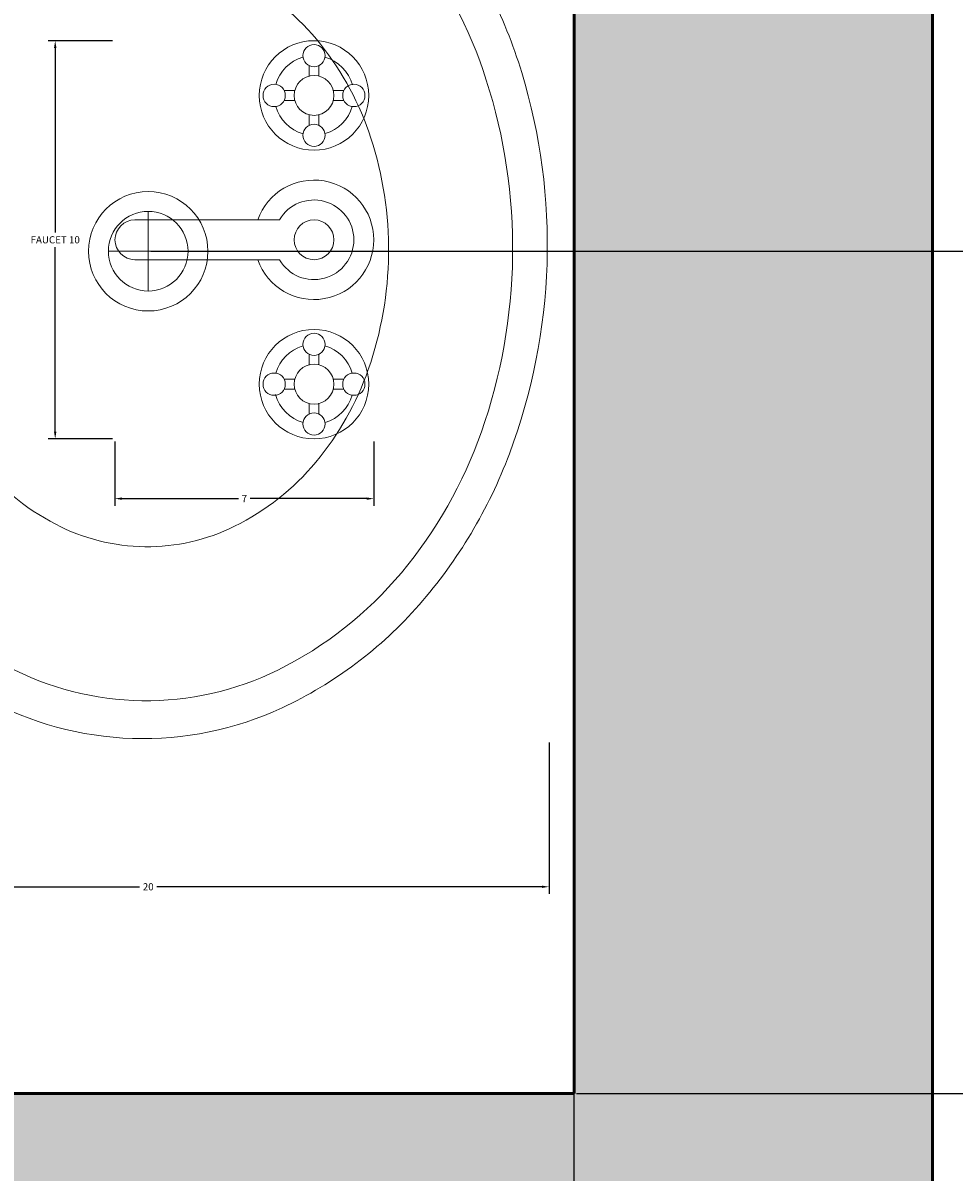
# Model space of a CAD drawing. Units: inches. Extents: x 2307 to 2544, y 2171 to 2540.
# Tile 42 of 52: x 2502 to 2525, y 2438 to 2466. Entities that reach past the tile are written whole.
import ezdxf

# ---------------------------------------------------------------- set-up
doc = ezdxf.new("R2010")
doc.units = ezdxf.units.IN
for name, color, linetype, lineweight in [('A-ANNO-DIMS', 2, 'Continuous', 18), ('A-FLOR-FIXT', 9, 'Continuous', 18), ('A-WALL', 7, 'Continuous', 50)]:
    doc.layers.add(name, color=color, linetype=linetype, lineweight=lineweight)
doc.layers.add('A-WALL-PATT', color=18, linetype='Continuous', lineweight=13, true_color=0x000000)
doc.styles.get("Standard").update_dxf_attribs({"font": 'arial.ttf'})
doc.dimstyles.get("Standard").update_dxf_attribs({"dimtxt": 0.18, "dimasz": 0.18, "dimexe": 0.18, "dimexo": 0.0625, "dimgap": 0.09, "dimtad": 0, "dimtih": 1, "dimtoh": 1, "dimdec": 4, "dimzin": 0, "dimdsep": 46, "dimtxsty": 'Standard', "dimcen": 0.09, "dimadec": 0, "dimazin": 0, "dimtfac": 1, "dimtdec": 4, "dimtofl": 0, "dimtmove": 0, "dimatfit": 3, "dimfxl": 1, "dimtolj": 1, "dimtzin": 0, "dimarcsym": 0})

# ---------------------------------------------------------------- blocks, each defined once
blk = doc.blocks.new('Sink - Oval top')
for p, q in [((0, 1), (0, -1)), ((-1, 0), (1, 0))]:
    blk.add_line(p, q)
for points in [[(-12.234, 0.394, 0.117634), (-11.465, -3.362, 0.104469), (-8.879, -6.804, 0.090016), (-5.083, -9.072, 0.08192), (-0.323, -10.016, 0.08192), (4.488, -9.381, 0.090016), (8.422, -7.361, 0.104469), (11.224, -4.093, 0.117634), (12.234, -0.394, 0.117634), (11.465, 3.362, 0.104469), (8.879, 6.804, 0.090016), (5.083, 9.072, 0.08192), (0.323, 10.016, 0.08192), (-4.488, 9.381, 0.090016), (-8.422, 7.361, 0.104469), (-11.224, 4.093, 0.117634)], [(-11.286, 0.159, 0.118622), (-10.516, -3.253, 0.104678), (-8.072, -6.359, 0.089562), (-4.538, -8.367, 0.081185), (-0.129, -9.152, 0.081185), (4.3, -8.492, 0.089562), (7.889, -6.584, 0.104678), (10.42, -3.548, 0.118622), (11.286, -0.159, 0.118622), (10.516, 3.253, 0.104678), (8.072, 6.359, 0.089562), (4.538, 8.367, 0.081185), (0.129, 9.152, 0.081185), (-4.3, 8.492, 0.089562), (-7.889, 6.584, 0.104678), (-10.42, 3.548, 0.118622)], [(-7.42, 0.083, 0.118283), (-6.907, -2.167, 0.104607), (-5.295, -4.21, 0.089718), (-2.967, -5.528, 0.081436), (-0.068, -6.037, 0.081436), (2.842, -5.593, 0.089718), (5.199, -4.327, 0.104607), (6.857, -2.321, 0.118283), (7.42, -0.083, 0.118283), (6.907, 2.167, 0.104607), (5.295, 4.21, 0.089718), (2.967, 5.528, 0.081436), (0.068, 6.037, 0.081436), (-2.842, 5.593, 0.089718), (-5.199, 4.327, 0.104607), (-6.857, 2.321, 0.118283)]]:
    blk.add_lwpolyline(points, format="xyb", close=True)
for radius in [1.5, 1]:
    blk.add_circle((0, 0), radius)
blk = doc.blocks.new('Faucet - Bathroom top')
for p, q in [((-3.75, 0.4788), (-3.75, 0.75)), ((-3.5, 0.482), (-3.5, 0.75)), ((3.5, 0.4788), (3.5, 0.75)), ((3.75, 0.482), (3.75, 0.75)), ((-4.107, 0.125), (-4.375, 0.125)), ((-3.1461, 0.125), (-2.875, 0.125)), ((3.143, 0.125), (2.875, 0.125)), ((4.1039, 0.125), (4.375, 0.125)), ((-4.1039, -0.125), (-4.375, -0.125)), ((-3.143, -0.125), (-2.875, -0.125)), ((3.1461, -0.125), (2.875, -0.125)), ((4.107, -0.125), (4.375, -0.125)), ((-3.75, -0.4821), (-3.75, -0.75)), ((-3.5, -0.4789), (-3.5, -0.75)), ((3.5, -0.4821), (3.5, -0.75)), ((3.75, -0.4789), (3.75, -0.75)), ((-0.5, -0.8639), (-0.5, -4.5)), ((0.5, -4.5), (0.5, -0.8631))]:
    blk.add_line(p, q)
for centre, radius in [((-3.625, 0), 1.375), ((-3.625, 1), 0.2795), ((3.625, 0), 1.375), ((3.625, 1), 0.2795), ((-3.625, 0), 0.5), ((0, 0), 0.5), ((3.625, 0), 0.5), ((-4.625, 0), 0.2795), ((-2.625, 0), 0.2795), ((2.625, 0), 0.2795), ((4.625, 0), 0.2795), ((-3.625, -1), 0.2795), ((3.625, -1), 0.2795)]:
    blk.add_circle(centre, radius)
for centre, radius, start, end in [((0, 0), 1.5, 289.6514, 250.3603), ((-3.625, 0), 1, 105.2407, 164.2093), ((-3.625, 0), 1, 16.44125, 74.07887), ((0, 0), 1, 300.3431, 239.7554), ((3.625, 0), 1, 106.12, 164.0884), ((3.625, 0), 1, 16.23422, 73.90469), ((-3.625, 0), 1, 196.2342, 253.9047), ((-3.625, 0), 1, 286.12, 344.0884), ((3.625, 0), 1, 196.4413, 254.0789), ((3.625, 0), 1, 285.2407, 344.2093), ((0, -4.5), 0.5, 180, 0)]:
    blk.add_arc(centre, radius, start, end)
blk = doc.blocks.new('*D23')
at = {"layer": 'A-ANNO-DIMS', "color": 0, "lineweight": -2, "transparency": 16777216}
for p, q in [((2494.934, 2448.317), (2494.934, 2444.517)), ((2515.07, 2448.317), (2515.07, 2444.517)), ((2495.114, 2444.697), (2504.782, 2444.697)), ((2514.89, 2444.697), (2505.222, 2444.697))]:
    blk.add_line(p, q, dxfattribs=at)
at = {"layer": 'A-ANNO-DIMS', "color": 0, "transparency": 16777216}
for points in [[(2495.114, 2444.727), (2495.114, 2444.667), (2494.934, 2444.697)], [(2514.89, 2444.727), (2514.89, 2444.667), (2515.07, 2444.697)]]:
    blk.add_solid(points, dxfattribs=at)
at = {"layer": 'Defpoints', "color": 0, "transparency": 16777216}
for p in [(2494.934, 2448.38), (2515.07, 2448.38), (2515.07, 2444.697)]:
    blk.add_point(p, dxfattribs=at)
at = {"layer": 'A-ANNO-DIMS', "color": 0, "transparency": 16777216, "insert": (2505.002, 2444.697), "char_height": 0.18, "attachment_point": 5}
blk.add_mtext('\\A1;20', dxfattribs=at)
blk = doc.blocks.new('*D24')
at = {"layer": 'A-ANNO-DIMS', "color": 0, "lineweight": -2, "transparency": 16777216}
for p, q in [((2504.104, 2465.943), (2502.486, 2465.943)), ((2502.666, 2465.763), (2502.666, 2461.126)), ((2502.666, 2456.123), (2502.666, 2460.76)), ((2504.104, 2455.943), (2502.486, 2455.943))]:
    blk.add_line(p, q, dxfattribs=at)
at = {"layer": 'A-ANNO-DIMS', "color": 0, "transparency": 16777216}
for points in [[(2502.636, 2465.763), (2502.696, 2465.763), (2502.666, 2465.943)], [(2502.636, 2456.123), (2502.696, 2456.123), (2502.666, 2455.943)]]:
    blk.add_solid(points, dxfattribs=at)
at = {"layer": 'Defpoints', "color": 0, "transparency": 16777216}
for p in [(2504.166, 2465.943), (2502.666, 2455.943), (2504.166, 2455.943)]:
    blk.add_point(p, dxfattribs=at)
at = {"layer": 'A-ANNO-DIMS', "color": 0, "transparency": 16777216, "insert": (2502.666, 2460.943), "char_height": 0.18, "attachment_point": 5}
blk.add_mtext('\\A1;FAUCET 10', dxfattribs=at)
blk = doc.blocks.new('*D25')
at = {"layer": 'A-ANNO-DIMS', "color": 0, "lineweight": -2, "transparency": 16777216}
for p, q in [((2504.166, 2455.88), (2504.166, 2454.263)), ((2510.666, 2455.88), (2510.666, 2454.263)), ((2504.346, 2454.443), (2507.268, 2454.443)), ((2510.486, 2454.443), (2507.565, 2454.443))]:
    blk.add_line(p, q, dxfattribs=at)
at = {"layer": 'A-ANNO-DIMS', "color": 0, "transparency": 16777216}
for points in [[(2504.346, 2454.473), (2504.346, 2454.413), (2504.166, 2454.443)], [(2510.486, 2454.473), (2510.486, 2454.413), (2510.666, 2454.443)]]:
    blk.add_solid(points, dxfattribs=at)
at = {"layer": 'Defpoints', "color": 0, "transparency": 16777216}
for p in [(2504.166, 2455.943), (2510.666, 2455.943), (2510.666, 2454.443)]:
    blk.add_point(p, dxfattribs=at)
at = {"layer": 'A-ANNO-DIMS', "color": 0, "transparency": 16777216, "insert": (2507.416, 2454.443), "char_height": 0.18, "attachment_point": 5}
blk.add_mtext('\\A1;7', dxfattribs=at)
blk = doc.blocks.new('*D37')
at = {"layer": 'A-ANNO-DIMS', "color": 0, "lineweight": -2, "transparency": 16777216}
for p, q in [((2524.758, 2520.51), (2544.026, 2520.51)), ((2543.846, 2520.33), (2543.846, 2355.692)), ((2543.846, 2190.69), (2543.846, 2355.328)), ((2524.758, 2190.51), (2544.026, 2190.51))]:
    blk.add_line(p, q, dxfattribs=at)
at = {"layer": 'A-ANNO-DIMS', "color": 0, "transparency": 16777216}
for points in [[(2543.816, 2520.33), (2543.876, 2520.33), (2543.846, 2520.51)], [(2543.816, 2190.69), (2543.876, 2190.69), (2543.846, 2190.51)]]:
    blk.add_solid(points, dxfattribs=at)
at = {"layer": 'Defpoints', "color": 0, "transparency": 16777216}
for p in [(2524.696, 2520.51), (2543.846, 2520.51), (2524.696, 2190.51)]:
    blk.add_point(p, dxfattribs=at)
at = {"layer": 'A-ANNO-DIMS', "color": 0, "transparency": 16777216, "insert": (2543.846, 2355.51), "char_height": 0.18, "attachment_point": 5}
blk.add_mtext('\\A1;330', dxfattribs=at)
blk = doc.blocks.new('*D61')
at = {"layer": 'A-ANNO-DIMS', "color": 0, "lineweight": -2, "transparency": 16777216}
for p, q in [((2491.696, 2435.572), (2491.696, 2540.345)), ((2515.696, 2435.572), (2515.696, 2540.345)), ((2491.876, 2540.165), (2503.476, 2540.165)), ((2515.516, 2540.165), (2503.916, 2540.165))]:
    blk.add_line(p, q, dxfattribs=at)
at = {"layer": 'A-ANNO-DIMS', "color": 0, "transparency": 16777216}
for points in [[(2491.876, 2540.195), (2491.876, 2540.135), (2491.696, 2540.165)], [(2515.516, 2540.195), (2515.516, 2540.135), (2515.696, 2540.165)]]:
    blk.add_solid(points, dxfattribs=at)
at = {"layer": 'Defpoints', "color": 0, "transparency": 16777216}
for p in [(2515.696, 2540.165), (2491.696, 2435.51), (2515.696, 2435.51)]:
    blk.add_point(p, dxfattribs=at)
at = {"layer": 'A-ANNO-DIMS', "color": 0, "transparency": 16777216, "insert": (2503.696, 2540.165), "char_height": 0.18, "attachment_point": 5}
blk.add_mtext('\\A1;24', dxfattribs=at)
blk = doc.blocks.new('*D63')
at = {"layer": 'A-ANNO-DIMS', "color": 0, "lineweight": -2, "transparency": 16777216}
for p, q in [((2505.065, 2460.655), (2544.026, 2460.655)), ((2543.846, 2460.475), (2543.846, 2450.264)), ((2543.846, 2439.69), (2543.846, 2449.9)), ((2515.758, 2439.51), (2544.026, 2439.51))]:
    blk.add_line(p, q, dxfattribs=at)
at = {"layer": 'A-ANNO-DIMS', "color": 0, "transparency": 16777216}
for points in [[(2543.816, 2460.475), (2543.876, 2460.475), (2543.846, 2460.655)], [(2543.816, 2439.69), (2543.876, 2439.69), (2543.846, 2439.51)]]:
    blk.add_solid(points, dxfattribs=at)
at = {"layer": 'Defpoints', "color": 0, "transparency": 16777216}
for p in [(2505.002, 2460.655), (2543.846, 2460.655), (2515.696, 2439.51)]:
    blk.add_point(p, dxfattribs=at)
at = {"layer": 'A-ANNO-DIMS', "color": 0, "transparency": 16777216, "insert": (2543.846, 2450.082), "char_height": 0.18, "attachment_point": 5}
blk.add_mtext('\\A1;21.145', dxfattribs=at)

msp = doc.modelspace()

# ---------------------------------------------------------------- hatches: boundary and pattern name
at = {"layer": 'A-WALL-PATT'}
h = msp.add_hatch(color=256, dxfattribs=at)
h.dxf.hatch_style = 1
h.paths.add_polyline_path([(2433.6935, 2199.5096), (2415.6423, 2199.5096), (2415.6423, 2190.5096), (2433.7832, 2190.5096)], flags=17)
h.paths.add_polyline_path([(2367.6423, 2199.5096), (2335.6958, 2199.5096), (2335.6958, 2307.3983), (2326.6958, 2307.3983), (2326.6958, 2190.5096), (2367.6423, 2190.5096)])
h.paths.add_polyline_path([(2524.6958, 2520.5096), (2496.7832, 2520.5096), (2496.7832, 2515.5149), (2472.7832, 2515.5149), (2472.7832, 2520.5096), (2415.4028, 2520.5096), (2415.4028, 2511.5096), (2451.6958, 2511.5096), (2451.6958, 2439.5096), (2451.6958, 2391.5096), (2445.6958, 2391.5096), (2445.6958, 2387.5096), (2455.6958, 2387.5096), (2455.6958, 2435.5096), (2461.6958, 2435.5096), (2461.6958, 2439.5096), (2455.6958, 2439.5096), (2455.6958, 2511.5096), (2515.6958, 2511.5096), (2515.6958, 2439.5096), (2491.6958, 2439.5096), (2491.6958, 2435.5096), (2515.6958, 2435.5096), (2515.6958, 2319.5096), (2451.6958, 2319.5096), (2451.6958, 2281.5096), (2481.6958, 2281.5096), (2481.6958, 2225.5096), (2485.6958, 2225.5096), (2485.6958, 2285.5096), (2455.6958, 2285.5096), (2455.6958, 2315.5096), (2515.6958, 2315.5096), (2515.6958, 2199.5096), (2469.6952, 2199.5096), (2469.785, 2190.5096), (2524.6958, 2190.5096)])

# ---------------------------------------------------------------- linework, layer by layer
at = {"layer": 'A-WALL'}
for p in [(2515.6958, 2511.5096), (2491.6958, 2439.5096)]:
    msp.add_line(p, (2515.6958, 2439.5096), dxfattribs=at)
msp.add_lwpolyline([(2433.7832, 2190.5096), (2326.6958, 2190.5096), (2326.6958, 2520.5096), (2524.6958, 2520.5096), (2524.6958, 2190.5096), (2469.785, 2190.5096)], dxfattribs=at)

# ---------------------------------------------------------------- block references
at = {"layer": 'A-FLOR-FIXT', "rotation": 270}
for name, p in [('Sink - Oval top', (2505.002, 2460.655)), ('Faucet - Bathroom top', (2509.1663, 2460.9426))]:
    msp.add_blockref(name, p, dxfattribs=at)

# ---------------------------------------------------------------- dimensions: what is measured, and where the dimension line sits
at = {"layer": 'A-ANNO-DIMS'}
for base, p1, p2, picture, middle in [((2515.6958, 2540.1649), (2491.6958, 2435.5096), (2515.6958, 2435.5096), '*D61', (2503.6958, 2540.1649)), ((2510.6664, 2454.4426), (2504.1663, 2455.9426), (2510.6664, 2455.9426), '*D25', (2507.4163, 2454.4426)), ((2515.0703, 2444.6969), (2494.9337, 2448.3795), (2515.0703, 2448.3795), '*D23', (2505.002, 2444.6969))]:
    dim = msp.add_linear_dim(base=base, p1=p1, p2=p2, dimstyle='Standard', override={"dimdec": 0, "dimlfac": 1, "dimrnd": 0, "dimzin": 0, "dimdsep": 46, "dimlunit": 2}, dxfattribs=at)
    dim.commit()
    dim.dimension.update_dxf_attribs({"geometry": picture, "text_midpoint": middle})
for base, p1, p2, override, picture, middle in [((2543.8458, 2520.5096), (2524.6958, 2190.5096), (2524.6958, 2520.5096), {"dimdec": 0, "dimlfac": 1, "dimrnd": 0, "dimzin": 0, "dimdsep": 46, "dimlunit": 2}, '*D37', (2543.8458, 2355.5096)), ((2543.8458, 2460.655), (2515.6958, 2439.5096), (2505.002, 2460.655), {"dimdec": 3, "dimlfac": 1, "dimrnd": 0, "dimzin": 0, "dimdsep": 46, "dimlunit": 2}, '*D63', (2543.8458, 2450.0823))]:
    dim = msp.add_linear_dim(base=base, p1=p1, p2=p2, angle=90, dimstyle='Standard', override=override, dxfattribs=at)
    dim.commit()
    dim.dimension.update_dxf_attribs({"geometry": picture, "text_midpoint": middle})
dim = msp.add_linear_dim(base=(2502.6663, 2455.9426), p1=(2504.1663, 2465.9426), p2=(2504.1663, 2455.9426), angle=270, text='FAUCET <>', dimstyle='Standard', override={"dimdec": 0, "dimlfac": 1, "dimrnd": 0, "dimzin": 0, "dimdsep": 46, "dimlunit": 2}, dxfattribs=at)
dim.commit()
dim.dimension.update_dxf_attribs({"geometry": '*D24', "text_midpoint": (2502.6663, 2460.9426)})

doc.saveas('drawing.dxf')
